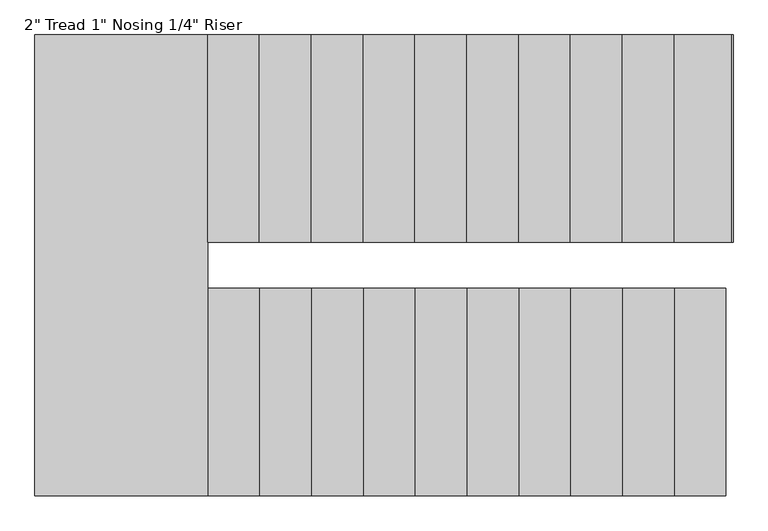
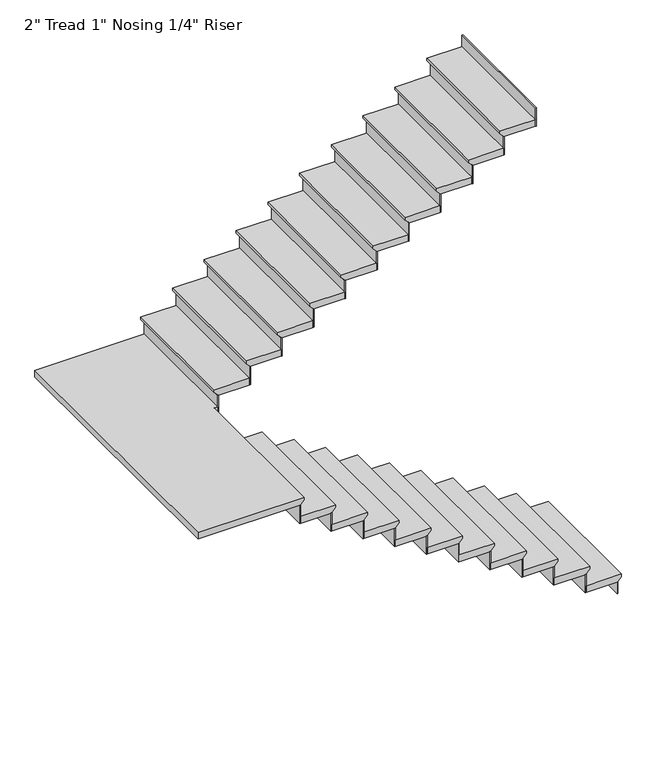
"""IFC4 building model written with IfcOpenShell, lengths in millimetres: stair flight geometry."""

from ifc_helpers import new_model, si_unit, origin, place, context, project, spatial, faceted_brep, source, transform, mapped, element, save


def stair_flight_ce5c0ca6(model_context):
    return source(origin(), model_context, "Body", "Brep", [
        faceted_brep([(-2080.8410855, 332.1803617, 3319.8954545), (-2080.8410855, 332.1803617, 3338.9454545), (-2080.8410855, -582.2196383, 3338.9454545), (-2080.8410855, -582.2196383, 3319.8954545), (-2106.2410855, 332.1803617, 3294.4954545), (-2106.2410855, -582.2196383, 3294.4954545), (-2334.8410855, 332.1803617, 3338.9454545), (-2334.8410855, -582.2196383, 3338.9454545), (-2106.2410855, -582.2196383, 3288.1454545), (-2334.8410855, -582.2196383, 3288.1454545), (-2334.8410855, 332.1803617, 3288.1454545), (-2106.2410855, 332.1803617, 3288.1454545)], [[[0, 1, 2, 3]], [[4, 0, 3, 5]], [[2, 1, 6, 7]], [[8, 9, 10, 11]], [[2, 7, 9, 8, 5, 3]], [[8, 11, 4, 5]], [[6, 1, 0, 4, 11, 10]], [[7, 6, 10, 9]]]),
        faceted_brep([(-2106.2410855, 332.1803617, 3288.1454545), (-2106.2410855, 332.1803617, 3200.4), (-2112.5910855, 332.1803617, 3200.4), (-2112.5910855, 332.1803617, 3288.1454545), (-2106.2410855, -582.2196383, 3288.1454545), (-2112.5910855, -582.2196383, 3288.1454545), (-2112.5910855, -582.2196383, 3200.4), (-2106.2410855, -582.2196383, 3200.4)], [[[0, 1, 2, 3]], [[4, 5, 6, 7]], [[1, 0, 4, 7]], [[2, 1, 7, 6]], [[3, 2, 6, 5]], [[0, 3, 5, 4]]]),
        faceted_brep([(-2334.8410855, 332.1803617, 3426.6909091), (-2334.8410855, 332.1803617, 3288.1454545), (-2341.1910855, 332.1803617, 3288.1454545), (-2341.1910855, 332.1803617, 3426.6909091), (-2334.8410855, -582.2196383, 3426.6909091), (-2341.1910855, -582.2196383, 3426.6909091), (-2341.1910855, -582.2196383, 3288.1454545), (-2334.8410855, -582.2196383, 3288.1454545)], [[[0, 1, 2, 3]], [[4, 5, 6, 7]], [[1, 0, 4, 7]], [[2, 1, 7, 6]], [[3, 2, 6, 5]], [[0, 3, 5, 4]]]),
        faceted_brep([(-2309.4410855, -582.2196383, 3477.4909091), (-2309.4410855, 332.1803617, 3477.4909091), (-2563.4410855, 332.1803617, 3477.4909091), (-2563.4410855, -582.2196383, 3477.4909091), (-2334.8410855, -582.2196383, 3426.6909091), (-2563.4410855, -582.2196383, 3426.6909091), (-2563.4410855, 332.1803617, 3426.6909091), (-2334.8410855, 332.1803617, 3426.6909091), (-2334.8410855, -582.2196383, 3433.0409091), (-2309.4410855, -582.2196383, 3458.4409091), (-2334.8410855, 332.1803617, 3433.0409091), (-2309.4410855, 332.1803617, 3458.4409091)], [[[0, 1, 2, 3]], [[4, 5, 6, 7]], [[0, 3, 5, 4, 8, 9]], [[4, 7, 10, 8]], [[2, 1, 11, 10, 7, 6]], [[3, 2, 6, 5]], [[11, 1, 0, 9]], [[10, 11, 9, 8]]]),
        faceted_brep([(-2563.4410855, 332.1803617, 3565.2363636), (-2563.4410855, 332.1803617, 3426.6909091), (-2569.7910855, 332.1803617, 3426.6909091), (-2569.7910855, 332.1803617, 3565.2363636), (-2563.4410855, -582.2196383, 3565.2363636), (-2569.7910855, -582.2196383, 3565.2363636), (-2569.7910855, -582.2196383, 3426.6909091), (-2563.4410855, -582.2196383, 3426.6909091)], [[[0, 1, 2, 3]], [[4, 5, 6, 7]], [[1, 0, 4, 7]], [[2, 1, 7, 6]], [[3, 2, 6, 5]], [[0, 3, 5, 4]]]),
        faceted_brep([(-2538.0410855, -582.2196383, 3616.0363636), (-2538.0410855, 332.1803617, 3616.0363636), (-2792.0410855, 332.1803617, 3616.0363636), (-2792.0410855, -582.2196383, 3616.0363636), (-2563.4410855, -582.2196383, 3565.2363636), (-2792.0410855, -582.2196383, 3565.2363636), (-2792.0410855, 332.1803617, 3565.2363636), (-2563.4410855, 332.1803617, 3565.2363636), (-2563.4410855, -582.2196383, 3571.5863636), (-2538.0410855, -582.2196383, 3596.9863636), (-2563.4410855, 332.1803617, 3571.5863636), (-2538.0410855, 332.1803617, 3596.9863636)], [[[0, 1, 2, 3]], [[4, 5, 6, 7]], [[0, 3, 5, 4, 8, 9]], [[4, 7, 10, 8]], [[2, 1, 11, 10, 7, 6]], [[3, 2, 6, 5]], [[11, 1, 0, 9]], [[10, 11, 9, 8]]]),
        faceted_brep([(-2792.0410855, 332.1803617, 3703.7818182), (-2792.0410855, 332.1803617, 3565.2363636), (-2798.3910855, 332.1803617, 3565.2363636), (-2798.3910855, 332.1803617, 3703.7818182), (-2792.0410855, -582.2196383, 3703.7818182), (-2798.3910855, -582.2196383, 3703.7818182), (-2798.3910855, -582.2196383, 3565.2363636), (-2792.0410855, -582.2196383, 3565.2363636)], [[[0, 1, 2, 3]], [[4, 5, 6, 7]], [[1, 0, 4, 7]], [[2, 1, 7, 6]], [[3, 2, 6, 5]], [[0, 3, 5, 4]]]),
        faceted_brep([(-2766.6410855, -582.2196383, 3754.5818182), (-2766.6410855, 332.1803617, 3754.5818182), (-3020.6410855, 332.1803617, 3754.5818182), (-3020.6410855, -582.2196383, 3754.5818182), (-2792.0410855, -582.2196383, 3703.7818182), (-3020.6410855, -582.2196383, 3703.7818182), (-3020.6410855, 332.1803617, 3703.7818182), (-2792.0410855, 332.1803617, 3703.7818182), (-2792.0410855, -582.2196383, 3710.1318182), (-2766.6410855, -582.2196383, 3735.5318182), (-2792.0410855, 332.1803617, 3710.1318182), (-2766.6410855, 332.1803617, 3735.5318182)], [[[0, 1, 2, 3]], [[4, 5, 6, 7]], [[0, 3, 5, 4, 8, 9]], [[4, 7, 10, 8]], [[2, 1, 11, 10, 7, 6]], [[3, 2, 6, 5]], [[11, 1, 0, 9]], [[10, 11, 9, 8]]]),
        faceted_brep([(-3020.6410855, 332.1803617, 3842.3272727), (-3020.6410855, 332.1803617, 3703.7818182), (-3026.9910855, 332.1803617, 3703.7818182), (-3026.9910855, 332.1803617, 3842.3272727), (-3020.6410855, -582.2196383, 3842.3272727), (-3026.9910855, -582.2196383, 3842.3272727), (-3026.9910855, -582.2196383, 3703.7818182), (-3020.6410855, -582.2196383, 3703.7818182)], [[[0, 1, 2, 3]], [[4, 5, 6, 7]], [[1, 0, 4, 7]], [[2, 1, 7, 6]], [[3, 2, 6, 5]], [[0, 3, 5, 4]]]),
        faceted_brep([(-2995.2410855, -582.2196383, 3893.1272727), (-2995.2410855, 332.1803617, 3893.1272727), (-3249.2410855, 332.1803617, 3893.1272727), (-3249.2410855, -582.2196383, 3893.1272727), (-3020.6410855, -582.2196383, 3842.3272727), (-3249.2410855, -582.2196383, 3842.3272727), (-3249.2410855, 332.1803617, 3842.3272727), (-3020.6410855, 332.1803617, 3842.3272727), (-3020.6410855, -582.2196383, 3848.6772727), (-2995.2410855, -582.2196383, 3874.0772727), (-3020.6410855, 332.1803617, 3848.6772727), (-2995.2410855, 332.1803617, 3874.0772727)], [[[0, 1, 2, 3]], [[4, 5, 6, 7]], [[0, 3, 5, 4, 8, 9]], [[4, 7, 10, 8]], [[2, 1, 11, 10, 7, 6]], [[3, 2, 6, 5]], [[11, 1, 0, 9]], [[10, 11, 9, 8]]]),
        faceted_brep([(-3249.2410855, 332.1803617, 3980.8727273), (-3249.2410855, 332.1803617, 3842.3272727), (-3255.5910855, 332.1803617, 3842.3272727), (-3255.5910855, 332.1803617, 3980.8727273), (-3249.2410855, -582.2196383, 3980.8727273), (-3255.5910855, -582.2196383, 3980.8727273), (-3255.5910855, -582.2196383, 3842.3272727), (-3249.2410855, -582.2196383, 3842.3272727)], [[[0, 1, 2, 3]], [[4, 5, 6, 7]], [[1, 0, 4, 7]], [[2, 1, 7, 6]], [[3, 2, 6, 5]], [[0, 3, 5, 4]]]),
        faceted_brep([(-3223.8410855, -582.2196383, 4031.6727273), (-3223.8410855, 332.1803617, 4031.6727273), (-3477.8410855, 332.1803617, 4031.6727273), (-3477.8410855, -582.2196383, 4031.6727273), (-3249.2410855, -582.2196383, 3980.8727273), (-3477.8410855, -582.2196383, 3980.8727273), (-3477.8410855, 332.1803617, 3980.8727273), (-3249.2410855, 332.1803617, 3980.8727273), (-3249.2410855, -582.2196383, 3987.2227273), (-3223.8410855, -582.2196383, 4012.6227273), (-3249.2410855, 332.1803617, 3987.2227273), (-3223.8410855, 332.1803617, 4012.6227273)], [[[0, 1, 2, 3]], [[4, 5, 6, 7]], [[0, 3, 5, 4, 8, 9]], [[4, 7, 10, 8]], [[2, 1, 11, 10, 7, 6]], [[3, 2, 6, 5]], [[11, 1, 0, 9]], [[10, 11, 9, 8]]]),
        faceted_brep([(-3477.8410855, 332.1803617, 4119.4181818), (-3477.8410855, 332.1803617, 3980.8727273), (-3484.1910855, 332.1803617, 3980.8727273), (-3484.1910855, 332.1803617, 4119.4181818), (-3477.8410855, -582.2196383, 4119.4181818), (-3484.1910855, -582.2196383, 4119.4181818), (-3484.1910855, -582.2196383, 3980.8727273), (-3477.8410855, -582.2196383, 3980.8727273)], [[[0, 1, 2, 3]], [[4, 5, 6, 7]], [[1, 0, 4, 7]], [[2, 1, 7, 6]], [[3, 2, 6, 5]], [[0, 3, 5, 4]]]),
        faceted_brep([(-3452.4410855, -582.2196383, 4170.2181818), (-3452.4410855, 332.1803617, 4170.2181818), (-3706.4410855, 332.1803617, 4170.2181818), (-3706.4410855, -582.2196383, 4170.2181818), (-3477.8410855, -582.2196383, 4119.4181818), (-3706.4410855, -582.2196383, 4119.4181818), (-3706.4410855, 332.1803617, 4119.4181818), (-3477.8410855, 332.1803617, 4119.4181818), (-3477.8410855, -582.2196383, 4125.7681818), (-3452.4410855, -582.2196383, 4151.1681818), (-3477.8410855, 332.1803617, 4125.7681818), (-3452.4410855, 332.1803617, 4151.1681818)], [[[0, 1, 2, 3]], [[4, 5, 6, 7]], [[0, 3, 5, 4, 8, 9]], [[4, 7, 10, 8]], [[2, 1, 11, 10, 7, 6]], [[3, 2, 6, 5]], [[11, 1, 0, 9]], [[10, 11, 9, 8]]]),
        faceted_brep([(-3706.4410855, 332.1803617, 4257.9636364), (-3706.4410855, 332.1803617, 4119.4181818), (-3712.7910855, 332.1803617, 4119.4181818), (-3712.7910855, 332.1803617, 4257.9636364), (-3706.4410855, -582.2196383, 4257.9636364), (-3712.7910855, -582.2196383, 4257.9636364), (-3712.7910855, -582.2196383, 4119.4181818), (-3706.4410855, -582.2196383, 4119.4181818)], [[[0, 1, 2, 3]], [[4, 5, 6, 7]], [[1, 0, 4, 7]], [[2, 1, 7, 6]], [[3, 2, 6, 5]], [[0, 3, 5, 4]]]),
        faceted_brep([(-3681.0410855, -582.2196383, 4308.7636364), (-3681.0410855, 332.1803617, 4308.7636364), (-3935.0410855, 332.1803617, 4308.7636364), (-3935.0410855, -582.2196383, 4308.7636364), (-3706.4410855, -582.2196383, 4257.9636364), (-3935.0410855, -582.2196383, 4257.9636364), (-3935.0410855, 332.1803617, 4257.9636364), (-3706.4410855, 332.1803617, 4257.9636364), (-3706.4410855, -582.2196383, 4264.3136364), (-3681.0410855, -582.2196383, 4289.7136364), (-3706.4410855, 332.1803617, 4264.3136364), (-3681.0410855, 332.1803617, 4289.7136364)], [[[0, 1, 2, 3]], [[4, 5, 6, 7]], [[0, 3, 5, 4, 8, 9]], [[4, 7, 10, 8]], [[2, 1, 11, 10, 7, 6]], [[3, 2, 6, 5]], [[11, 1, 0, 9]], [[10, 11, 9, 8]]]),
        faceted_brep([(-3935.0410855, 332.1803617, 4396.5090909), (-3935.0410855, 332.1803617, 4257.9636364), (-3941.3910855, 332.1803617, 4257.9636364), (-3941.3910855, 332.1803617, 4396.5090909), (-3935.0410855, -582.2196383, 4396.5090909), (-3941.3910855, -582.2196383, 4396.5090909), (-3941.3910855, -582.2196383, 4257.9636364), (-3935.0410855, -582.2196383, 4257.9636364)], [[[0, 1, 2, 3]], [[4, 5, 6, 7]], [[1, 0, 4, 7]], [[2, 1, 7, 6]], [[3, 2, 6, 5]], [[0, 3, 5, 4]]]),
        faceted_brep([(-3909.6410855, -582.2196383, 4447.3090909), (-3909.6410855, 332.1803617, 4447.3090909), (-4163.6410855, 332.1803617, 4447.3090909), (-4163.6410855, -582.2196383, 4447.3090909), (-3935.0410855, -582.2196383, 4396.5090909), (-4163.6410855, -582.2196383, 4396.5090909), (-4163.6410855, 332.1803617, 4396.5090909), (-3935.0410855, 332.1803617, 4396.5090909), (-3935.0410855, -582.2196383, 4402.8590909), (-3909.6410855, -582.2196383, 4428.2590909), (-3935.0410855, 332.1803617, 4402.8590909), (-3909.6410855, 332.1803617, 4428.2590909)], [[[0, 1, 2, 3]], [[4, 5, 6, 7]], [[0, 3, 5, 4, 8, 9]], [[4, 7, 10, 8]], [[2, 1, 11, 10, 7, 6]], [[3, 2, 6, 5]], [[11, 1, 0, 9]], [[10, 11, 9, 8]]]),
        faceted_brep([(-4163.6410855, 332.1803617, 4535.0545455), (-4163.6410855, 332.1803617, 4396.5090909), (-4169.9910855, 332.1803617, 4396.5090909), (-4169.9910855, 332.1803617, 4535.0545455), (-4163.6410855, -582.2196383, 4535.0545455), (-4169.9910855, -582.2196383, 4535.0545455), (-4169.9910855, -582.2196383, 4396.5090909), (-4163.6410855, -582.2196383, 4396.5090909)], [[[0, 1, 2, 3]], [[4, 5, 6, 7]], [[1, 0, 4, 7]], [[2, 1, 7, 6]], [[3, 2, 6, 5]], [[0, 3, 5, 4]]]),
        faceted_brep([(-4138.2410855, -582.2196383, 4585.8545455), (-4138.2410855, 332.1803617, 4585.8545455), (-4392.2410855, 332.1803617, 4585.8545455), (-4392.2410855, -582.2196383, 4585.8545455), (-4163.6410855, -582.2196383, 4535.0545455), (-4392.2410855, -582.2196383, 4535.0545455), (-4392.2410855, 332.1803617, 4535.0545455), (-4163.6410855, 332.1803617, 4535.0545455), (-4163.6410855, -582.2196383, 4541.4045455), (-4138.2410855, -582.2196383, 4566.8045455), (-4163.6410855, 332.1803617, 4541.4045455), (-4138.2410855, 332.1803617, 4566.8045455)], [[[0, 1, 2, 3]], [[4, 5, 6, 7]], [[0, 3, 5, 4, 8, 9]], [[4, 7, 10, 8]], [[2, 1, 11, 10, 7, 6]], [[3, 2, 6, 5]], [[11, 1, 0, 9]], [[10, 11, 9, 8]]]),
        faceted_brep([(-4392.2410855, 332.1803617, 4673.6), (-4392.2410855, 332.1803617, 4535.0545455), (-4398.5910855, 332.1803617, 4535.0545455), (-4398.5910855, 332.1803617, 4673.6), (-4392.2410855, -582.2196383, 4673.6), (-4398.5910855, -582.2196383, 4673.6), (-4398.5910855, -582.2196383, 4535.0545455), (-4392.2410855, -582.2196383, 4535.0545455)], [[[0, 1, 2, 3]], [[4, 5, 6, 7]], [[1, 0, 4, 7]], [[2, 1, 7, 6]], [[3, 2, 6, 5]], [[0, 3, 5, 4]]]),
        faceted_brep([(-4341.4410855, 1449.7803617, 4724.4), (-5128.8410855, 1449.7803617, 4724.4), (-5128.8410855, -582.2196383, 4724.4), (-4366.8410855, -582.2196383, 4724.4), (-4366.8410855, 535.3803617, 4724.4), (-4341.4410855, 535.3803617, 4724.4), (-5128.8410855, 1449.7803617, 4673.6), (-4341.4410855, 1449.7803617, 4673.6), (-4341.4410855, 535.3803617, 4673.6), (-4366.8410855, 535.3803617, 4673.6), (-4366.8410855, 332.1803617, 4673.6), (-4392.2410855, 332.1803617, 4673.6), (-4392.2410855, -582.2196383, 4673.6), (-5128.8410855, -582.2196383, 4673.6), (-4392.2410855, -582.2196383, 4679.95), (-4366.8410855, -582.2196383, 4705.35), (-4392.2410855, 332.1803617, 4679.95), (-4366.8410855, 332.1803617, 4705.35)], [[[0, 1, 2, 3, 4, 5]], [[6, 7, 8, 9, 10, 11, 12, 13]], [[1, 0, 7, 6]], [[2, 1, 6, 13]], [[3, 2, 13, 12, 14, 15]], [[12, 11, 16, 14]], [[11, 10, 17, 16]], [[4, 3, 15, 17, 10, 9]], [[5, 4, 9, 8]], [[0, 5, 8, 7]], [[15, 14, 16, 17]]]),
        faceted_brep([(-4341.4410855, 535.3803617, 4812.1454545), (-4341.4410855, 535.3803617, 4673.6), (-4335.0910855, 535.3803617, 4673.6), (-4335.0910855, 535.3803617, 4812.1454545), (-4341.4410855, 1449.7803617, 4812.1454545), (-4335.0910855, 1449.7803617, 4812.1454545), (-4335.0910855, 1449.7803617, 4673.6), (-4341.4410855, 1449.7803617, 4673.6)], [[[0, 1, 2, 3]], [[4, 5, 6, 7]], [[1, 0, 4, 7]], [[2, 1, 7, 6]], [[3, 2, 6, 5]], [[0, 3, 5, 4]]]),
        faceted_brep([(-4366.8410855, 1449.7803617, 4862.9454545), (-4366.8410855, 535.3803617, 4862.9454545), (-4112.8410855, 535.3803617, 4862.9454545), (-4112.8410855, 1449.7803617, 4862.9454545), (-4341.4410855, 1449.7803617, 4812.1454545), (-4112.8410855, 1449.7803617, 4812.1454545), (-4112.8410855, 535.3803617, 4812.1454545), (-4341.4410855, 535.3803617, 4812.1454545), (-4341.4410855, 1449.7803617, 4818.4954545), (-4366.8410855, 1449.7803617, 4843.8954545), (-4341.4410855, 535.3803617, 4818.4954545), (-4366.8410855, 535.3803617, 4843.8954545)], [[[0, 1, 2, 3]], [[4, 5, 6, 7]], [[0, 3, 5, 4, 8, 9]], [[4, 7, 10, 8]], [[2, 1, 11, 10, 7, 6]], [[3, 2, 6, 5]], [[11, 1, 0, 9]], [[10, 11, 9, 8]]]),
        faceted_brep([(-4112.8410855, 535.3803617, 4950.6909091), (-4112.8410855, 535.3803617, 4812.1454545), (-4106.4910855, 535.3803617, 4812.1454545), (-4106.4910855, 535.3803617, 4950.6909091), (-4112.8410855, 1449.7803617, 4950.6909091), (-4106.4910855, 1449.7803617, 4950.6909091), (-4106.4910855, 1449.7803617, 4812.1454545), (-4112.8410855, 1449.7803617, 4812.1454545)], [[[0, 1, 2, 3]], [[4, 5, 6, 7]], [[1, 0, 4, 7]], [[2, 1, 7, 6]], [[3, 2, 6, 5]], [[0, 3, 5, 4]]]),
        faceted_brep([(-4138.2410855, 1449.7803617, 5001.4909091), (-4138.2410855, 535.3803617, 5001.4909091), (-3884.2410855, 535.3803617, 5001.4909091), (-3884.2410855, 1449.7803617, 5001.4909091), (-4112.8410855, 1449.7803617, 4950.6909091), (-3884.2410855, 1449.7803617, 4950.6909091), (-3884.2410855, 535.3803617, 4950.6909091), (-4112.8410855, 535.3803617, 4950.6909091), (-4112.8410855, 1449.7803617, 4957.0409091), (-4138.2410855, 1449.7803617, 4982.4409091), (-4112.8410855, 535.3803617, 4957.0409091), (-4138.2410855, 535.3803617, 4982.4409091)], [[[0, 1, 2, 3]], [[4, 5, 6, 7]], [[0, 3, 5, 4, 8, 9]], [[4, 7, 10, 8]], [[2, 1, 11, 10, 7, 6]], [[3, 2, 6, 5]], [[11, 1, 0, 9]], [[10, 11, 9, 8]]]),
        faceted_brep([(-3884.2410855, 535.3803617, 5089.2363636), (-3884.2410855, 535.3803617, 4950.6909091), (-3877.8910855, 535.3803617, 4950.6909091), (-3877.8910855, 535.3803617, 5089.2363636), (-3884.2410855, 1449.7803617, 5089.2363636), (-3877.8910855, 1449.7803617, 5089.2363636), (-3877.8910855, 1449.7803617, 4950.6909091), (-3884.2410855, 1449.7803617, 4950.6909091)], [[[0, 1, 2, 3]], [[4, 5, 6, 7]], [[1, 0, 4, 7]], [[2, 1, 7, 6]], [[3, 2, 6, 5]], [[0, 3, 5, 4]]]),
        faceted_brep([(-3909.6410855, 1449.7803617, 5140.0363636), (-3909.6410855, 535.3803617, 5140.0363636), (-3655.6410855, 535.3803617, 5140.0363636), (-3655.6410855, 1449.7803617, 5140.0363636), (-3884.2410855, 1449.7803617, 5089.2363636), (-3655.6410855, 1449.7803617, 5089.2363636), (-3655.6410855, 535.3803617, 5089.2363636), (-3884.2410855, 535.3803617, 5089.2363636), (-3884.2410855, 1449.7803617, 5095.5863636), (-3909.6410855, 1449.7803617, 5120.9863636), (-3884.2410855, 535.3803617, 5095.5863636), (-3909.6410855, 535.3803617, 5120.9863636)], [[[0, 1, 2, 3]], [[4, 5, 6, 7]], [[0, 3, 5, 4, 8, 9]], [[4, 7, 10, 8]], [[2, 1, 11, 10, 7, 6]], [[3, 2, 6, 5]], [[11, 1, 0, 9]], [[10, 11, 9, 8]]]),
        faceted_brep([(-3655.6410855, 535.3803617, 5227.7818182), (-3655.6410855, 535.3803617, 5089.2363636), (-3649.2910855, 535.3803617, 5089.2363636), (-3649.2910855, 535.3803617, 5227.7818182), (-3655.6410855, 1449.7803617, 5227.7818182), (-3649.2910855, 1449.7803617, 5227.7818182), (-3649.2910855, 1449.7803617, 5089.2363636), (-3655.6410855, 1449.7803617, 5089.2363636)], [[[0, 1, 2, 3]], [[4, 5, 6, 7]], [[1, 0, 4, 7]], [[2, 1, 7, 6]], [[3, 2, 6, 5]], [[0, 3, 5, 4]]]),
        faceted_brep([(-3681.0410855, 1449.7803617, 5278.5818182), (-3681.0410855, 535.3803617, 5278.5818182), (-3427.0410855, 535.3803617, 5278.5818182), (-3427.0410855, 1449.7803617, 5278.5818182), (-3655.6410855, 1449.7803617, 5227.7818182), (-3427.0410855, 1449.7803617, 5227.7818182), (-3427.0410855, 535.3803617, 5227.7818182), (-3655.6410855, 535.3803617, 5227.7818182), (-3655.6410855, 1449.7803617, 5234.1318182), (-3681.0410855, 1449.7803617, 5259.5318182), (-3655.6410855, 535.3803617, 5234.1318182), (-3681.0410855, 535.3803617, 5259.5318182)], [[[0, 1, 2, 3]], [[4, 5, 6, 7]], [[0, 3, 5, 4, 8, 9]], [[4, 7, 10, 8]], [[2, 1, 11, 10, 7, 6]], [[3, 2, 6, 5]], [[11, 1, 0, 9]], [[10, 11, 9, 8]]]),
        faceted_brep([(-3427.0410855, 535.3803617, 5366.3272727), (-3427.0410855, 535.3803617, 5227.7818182), (-3420.6910855, 535.3803617, 5227.7818182), (-3420.6910855, 535.3803617, 5366.3272727), (-3427.0410855, 1449.7803617, 5366.3272727), (-3420.6910855, 1449.7803617, 5366.3272727), (-3420.6910855, 1449.7803617, 5227.7818182), (-3427.0410855, 1449.7803617, 5227.7818182)], [[[0, 1, 2, 3]], [[4, 5, 6, 7]], [[1, 0, 4, 7]], [[2, 1, 7, 6]], [[3, 2, 6, 5]], [[0, 3, 5, 4]]]),
        faceted_brep([(-3452.4410855, 1449.7803617, 5417.1272727), (-3452.4410855, 535.3803617, 5417.1272727), (-3198.4410855, 535.3803617, 5417.1272727), (-3198.4410855, 1449.7803617, 5417.1272727), (-3427.0410855, 1449.7803617, 5366.3272727), (-3198.4410855, 1449.7803617, 5366.3272727), (-3198.4410855, 535.3803617, 5366.3272727), (-3427.0410855, 535.3803617, 5366.3272727), (-3427.0410855, 1449.7803617, 5372.6772727), (-3452.4410855, 1449.7803617, 5398.0772727), (-3427.0410855, 535.3803617, 5372.6772727), (-3452.4410855, 535.3803617, 5398.0772727)], [[[0, 1, 2, 3]], [[4, 5, 6, 7]], [[0, 3, 5, 4, 8, 9]], [[4, 7, 10, 8]], [[2, 1, 11, 10, 7, 6]], [[3, 2, 6, 5]], [[11, 1, 0, 9]], [[10, 11, 9, 8]]]),
        faceted_brep([(-3198.4410855, 535.3803617, 5504.8727273), (-3198.4410855, 535.3803617, 5366.3272727), (-3192.0910855, 535.3803617, 5366.3272727), (-3192.0910855, 535.3803617, 5504.8727273), (-3198.4410855, 1449.7803617, 5504.8727273), (-3192.0910855, 1449.7803617, 5504.8727273), (-3192.0910855, 1449.7803617, 5366.3272727), (-3198.4410855, 1449.7803617, 5366.3272727)], [[[0, 1, 2, 3]], [[4, 5, 6, 7]], [[1, 0, 4, 7]], [[2, 1, 7, 6]], [[3, 2, 6, 5]], [[0, 3, 5, 4]]]),
        faceted_brep([(-3223.8410855, 1449.7803617, 5555.6727273), (-3223.8410855, 535.3803617, 5555.6727273), (-2969.8410855, 535.3803617, 5555.6727273), (-2969.8410855, 1449.7803617, 5555.6727273), (-3198.4410855, 1449.7803617, 5504.8727273), (-2969.8410855, 1449.7803617, 5504.8727273), (-2969.8410855, 535.3803617, 5504.8727273), (-3198.4410855, 535.3803617, 5504.8727273), (-3198.4410855, 1449.7803617, 5511.2227273), (-3223.8410855, 1449.7803617, 5536.6227273), (-3198.4410855, 535.3803617, 5511.2227273), (-3223.8410855, 535.3803617, 5536.6227273)], [[[0, 1, 2, 3]], [[4, 5, 6, 7]], [[0, 3, 5, 4, 8, 9]], [[4, 7, 10, 8]], [[2, 1, 11, 10, 7, 6]], [[3, 2, 6, 5]], [[11, 1, 0, 9]], [[10, 11, 9, 8]]]),
        faceted_brep([(-2969.8410855, 535.3803617, 5643.4181818), (-2969.8410855, 535.3803617, 5504.8727273), (-2963.4910855, 535.3803617, 5504.8727273), (-2963.4910855, 535.3803617, 5643.4181818), (-2969.8410855, 1449.7803617, 5643.4181818), (-2963.4910855, 1449.7803617, 5643.4181818), (-2963.4910855, 1449.7803617, 5504.8727273), (-2969.8410855, 1449.7803617, 5504.8727273)], [[[0, 1, 2, 3]], [[4, 5, 6, 7]], [[1, 0, 4, 7]], [[2, 1, 7, 6]], [[3, 2, 6, 5]], [[0, 3, 5, 4]]]),
        faceted_brep([(-2995.2410855, 1449.7803617, 5694.2181818), (-2995.2410855, 535.3803617, 5694.2181818), (-2741.2410855, 535.3803617, 5694.2181818), (-2741.2410855, 1449.7803617, 5694.2181818), (-2969.8410855, 1449.7803617, 5643.4181818), (-2741.2410855, 1449.7803617, 5643.4181818), (-2741.2410855, 535.3803617, 5643.4181818), (-2969.8410855, 535.3803617, 5643.4181818), (-2969.8410855, 1449.7803617, 5649.7681818), (-2995.2410855, 1449.7803617, 5675.1681818), (-2969.8410855, 535.3803617, 5649.7681818), (-2995.2410855, 535.3803617, 5675.1681818)], [[[0, 1, 2, 3]], [[4, 5, 6, 7]], [[0, 3, 5, 4, 8, 9]], [[4, 7, 10, 8]], [[2, 1, 11, 10, 7, 6]], [[3, 2, 6, 5]], [[11, 1, 0, 9]], [[10, 11, 9, 8]]]),
        faceted_brep([(-2741.2410855, 535.3803617, 5781.9636364), (-2741.2410855, 535.3803617, 5643.4181818), (-2734.8910855, 535.3803617, 5643.4181818), (-2734.8910855, 535.3803617, 5781.9636364), (-2741.2410855, 1449.7803617, 5781.9636364), (-2734.8910855, 1449.7803617, 5781.9636364), (-2734.8910855, 1449.7803617, 5643.4181818), (-2741.2410855, 1449.7803617, 5643.4181818)], [[[0, 1, 2, 3]], [[4, 5, 6, 7]], [[1, 0, 4, 7]], [[2, 1, 7, 6]], [[3, 2, 6, 5]], [[0, 3, 5, 4]]]),
        faceted_brep([(-2766.6410855, 1449.7803617, 5832.7636364), (-2766.6410855, 535.3803617, 5832.7636364), (-2512.6410855, 535.3803617, 5832.7636364), (-2512.6410855, 1449.7803617, 5832.7636364), (-2741.2410855, 1449.7803617, 5781.9636364), (-2512.6410855, 1449.7803617, 5781.9636364), (-2512.6410855, 535.3803617, 5781.9636364), (-2741.2410855, 535.3803617, 5781.9636364), (-2741.2410855, 1449.7803617, 5788.3136364), (-2766.6410855, 1449.7803617, 5813.7136364), (-2741.2410855, 535.3803617, 5788.3136364), (-2766.6410855, 535.3803617, 5813.7136364)], [[[0, 1, 2, 3]], [[4, 5, 6, 7]], [[0, 3, 5, 4, 8, 9]], [[4, 7, 10, 8]], [[2, 1, 11, 10, 7, 6]], [[3, 2, 6, 5]], [[11, 1, 0, 9]], [[10, 11, 9, 8]]]),
        faceted_brep([(-2512.6410855, 535.3803617, 5920.5090909), (-2512.6410855, 535.3803617, 5781.9636364), (-2506.2910855, 535.3803617, 5781.9636364), (-2506.2910855, 535.3803617, 5920.5090909), (-2512.6410855, 1449.7803617, 5920.5090909), (-2506.2910855, 1449.7803617, 5920.5090909), (-2506.2910855, 1449.7803617, 5781.9636364), (-2512.6410855, 1449.7803617, 5781.9636364)], [[[0, 1, 2, 3]], [[4, 5, 6, 7]], [[1, 0, 4, 7]], [[2, 1, 7, 6]], [[3, 2, 6, 5]], [[0, 3, 5, 4]]]),
        faceted_brep([(-2538.0410855, 1449.7803617, 5971.3090909), (-2538.0410855, 535.3803617, 5971.3090909), (-2284.0410855, 535.3803617, 5971.3090909), (-2284.0410855, 1449.7803617, 5971.3090909), (-2512.6410855, 1449.7803617, 5920.5090909), (-2284.0410855, 1449.7803617, 5920.5090909), (-2284.0410855, 535.3803617, 5920.5090909), (-2512.6410855, 535.3803617, 5920.5090909), (-2512.6410855, 1449.7803617, 5926.8590909), (-2538.0410855, 1449.7803617, 5952.2590909), (-2512.6410855, 535.3803617, 5926.8590909), (-2538.0410855, 535.3803617, 5952.2590909)], [[[0, 1, 2, 3]], [[4, 5, 6, 7]], [[0, 3, 5, 4, 8, 9]], [[4, 7, 10, 8]], [[2, 1, 11, 10, 7, 6]], [[3, 2, 6, 5]], [[11, 1, 0, 9]], [[10, 11, 9, 8]]]),
        faceted_brep([(-2284.0410855, 535.3803617, 6059.0545455), (-2284.0410855, 535.3803617, 5920.5090909), (-2277.6910855, 535.3803617, 5920.5090909), (-2277.6910855, 535.3803617, 6059.0545455), (-2284.0410855, 1449.7803617, 6059.0545455), (-2277.6910855, 1449.7803617, 6059.0545455), (-2277.6910855, 1449.7803617, 5920.5090909), (-2284.0410855, 1449.7803617, 5920.5090909)], [[[0, 1, 2, 3]], [[4, 5, 6, 7]], [[1, 0, 4, 7]], [[2, 1, 7, 6]], [[3, 2, 6, 5]], [[0, 3, 5, 4]]]),
        faceted_brep([(-2055.4410855, 535.3803617, 6197.6), (-2055.4410855, 535.3803617, 6059.0545455), (-2049.0910855, 535.3803617, 6059.0545455), (-2049.0910855, 535.3803617, 6197.6), (-2055.4410855, 1449.7803617, 6197.6), (-2049.0910855, 1449.7803617, 6197.6), (-2049.0910855, 1449.7803617, 6059.0545455), (-2055.4410855, 1449.7803617, 6059.0545455)], [[[0, 1, 2, 3]], [[4, 5, 6, 7]], [[1, 0, 4, 7]], [[2, 1, 7, 6]], [[3, 2, 6, 5]], [[0, 3, 5, 4]]]),
        faceted_brep([(-2309.4410855, 1449.7803617, 6109.8545455), (-2309.4410855, 535.3803617, 6109.8545455), (-2055.4410855, 535.3803617, 6109.8545455), (-2055.4410855, 1449.7803617, 6109.8545455), (-2284.0410855, 1449.7803617, 6059.0545455), (-2055.4410855, 1449.7803617, 6059.0545455), (-2055.4410855, 535.3803617, 6059.0545455), (-2284.0410855, 535.3803617, 6059.0545455), (-2284.0410855, 1449.7803617, 6065.4045455), (-2309.4410855, 1449.7803617, 6090.8045455), (-2284.0410855, 535.3803617, 6065.4045455), (-2309.4410855, 535.3803617, 6090.8045455)], [[[0, 1, 2, 3]], [[4, 5, 6, 7]], [[0, 3, 5, 4, 8, 9]], [[4, 7, 10, 8]], [[2, 1, 11, 10, 7, 6]], [[3, 2, 6, 5]], [[11, 1, 0, 9]], [[10, 11, 9, 8]]]),
    ])


if __name__ == "__main__":
    model = new_model("IFC4")
    model_context = context("Model", 3, world=origin())
    ifc_project = project(units=[si_unit("LENGTHUNIT", "METRE", prefix="MILLI")], contexts=[model_context])
    site = spatial("IfcSite", under=ifc_project)
    building = spatial("IfcBuilding", under=site)
    placement = place(None, origin())
    stair_flight_shape = stair_flight_ce5c0ca6(model_context)
    element("IfcStairFlight", 1, ObjectType="2\" Tread 1\" Nosing 1/4\" Riser", at=placement, inside=building, context=model_context, shape_type="MappedRepresentation", body=[
        mapped(stair_flight_shape, transform((0.0, 0.0, 0.0), x_axis=(1.0, 0.0, 0.0), y_axis=(0.0, 1.0, 0.0), z_axis=(0.0, 0.0, 1.0))),
    ])
    save(model, "model.ifc")
